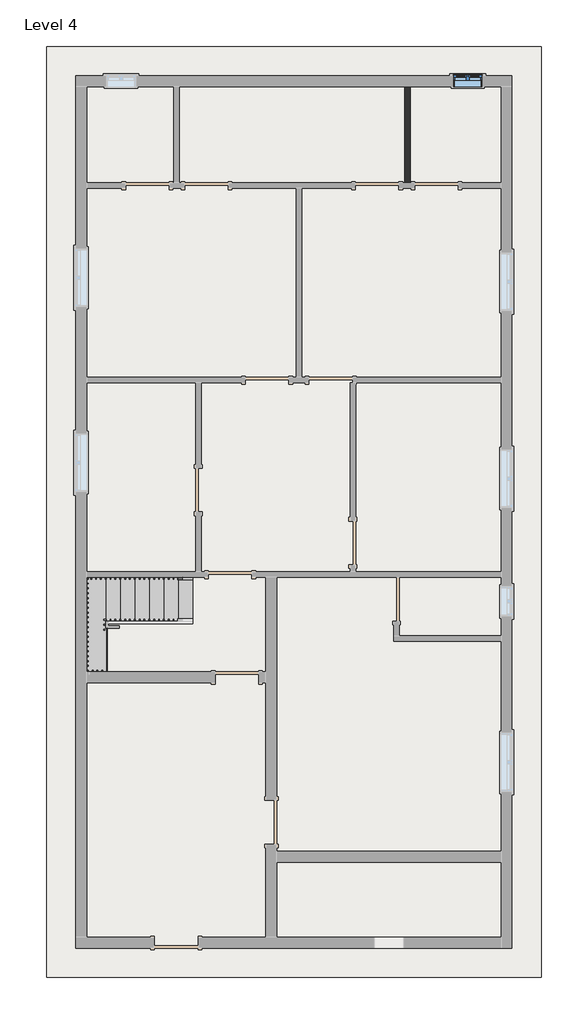
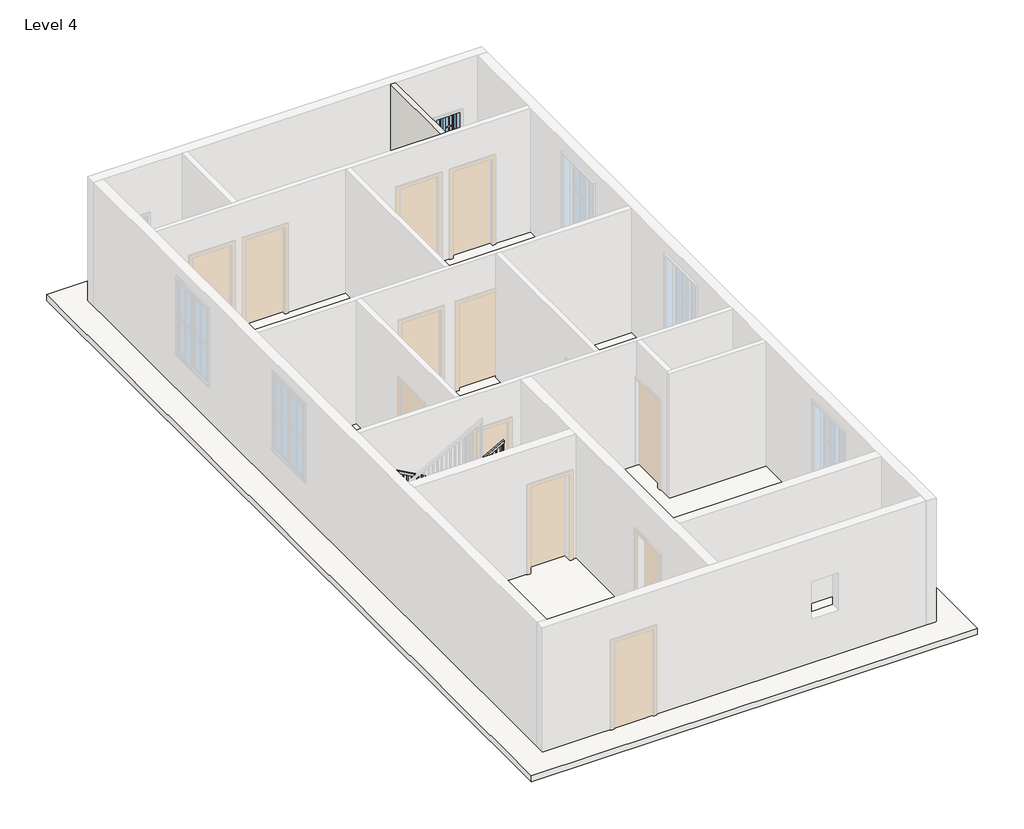
# One storey, part 2 of 3: 1 railing, 1 slab, 1 stair flight, 1 wall, 1 window.
"""IFC4 building model written with IfcOpenShell, lengths in millimetres."""

from ifc_helpers import new_model, si_unit, frame, origin, place, context, project, spatial, polyline, outline, extrude, faceted_brep, transform, mapped, element, save
from components import stair_flight_ac649a0f, window_c417fced

model = new_model("IFC4")

# Units and contexts
model_context = context("Model", 3, world=origin())
ifc_project = project(units=[si_unit("LENGTHUNIT", "METRE", prefix="MILLI")], contexts=[model_context])

# Site, building, storey
site = spatial("IfcSite", under=ifc_project)
building = spatial("IfcBuilding", under=site)
storey = spatial("IfcBuildingStorey", under=building, Name="Level 4", Elevation=9144.0)

# Railing
placement = place(None, origin())
element("IfcRailing", 1, ObjectType="Handrail - Rectangular", at=placement, inside=storey, context=model_context, shape_type="SolidModel", body=[
    faceted_brep([(3727.9146873, 3657.6, 10227.7333333), (3727.9146873, 3657.6, 10169.620221), (3727.9146873, 3708.4, 10169.620221), (3727.9146873, 3708.4, 10227.7333333), (1899.1146873, 3657.6, 11243.7333333), (1885.9510851, 3657.6, 11192.9333333), (1885.9510851, 3708.4, 11192.9333333), (1899.1146873, 3708.4, 11243.7333333), (1549.4, 3657.6, 11243.7333333), (1549.4, 3657.6, 11192.9333333), (1498.6, 3708.4, 11192.9333333), (1498.6, 3708.4, 11243.7333333), (1549.4, 1778.0, 11243.7333333), (1549.4, 1778.0, 11192.9333333), (1498.6, 1727.2, 11192.9333333), (1498.6, 1727.2, 11243.7333333), (1594.3146873, 1778.0, 11243.7333333), (1607.4782895, 1778.0, 11192.9333333), (1607.4782895, 1727.2, 11192.9333333), (1594.3146873, 1727.2, 11243.7333333), (3727.9146873, 1778.0, 12429.0666667), (3727.9146873, 1727.2, 12429.0666667), (3727.9146873, 1727.2, 12370.9535543), (3727.9146873, 1778.0, 12370.9535543)], [[[0, 1, 2, 3]], [[1, 0, 4, 5]], [[2, 1, 5, 6]], [[3, 2, 6, 7]], [[0, 3, 7, 4]], [[5, 4, 8, 9]], [[6, 5, 9, 10]], [[7, 6, 10, 11]], [[4, 7, 11, 8]], [[9, 8, 12, 13]], [[10, 9, 13, 14]], [[11, 10, 14, 15]], [[8, 11, 15, 12]], [[13, 12, 16, 17]], [[14, 13, 17, 18]], [[15, 14, 18, 19]], [[12, 15, 19, 16]], [[20, 21, 22, 23]], [[17, 16, 20, 23]], [[18, 17, 23, 22]], [[19, 18, 22, 21]], [[16, 19, 21, 20]]]),
    extrude(outline(polyline([(12337.1815058, 3667.125), (12326.5981725, 3648.075), (11345.3333333, 3648.075), (11345.3333333, 3667.125), (12337.1815058, 3667.125)])), frame((0.0, 1743.075, 0.0), z_axis=(0.0, 1.0, 0.0), x_axis=(0.0, 0.0, 1.0)), (0.0, 0.0, 1.0), 19.05),
    extrude(outline(polyline([(12280.7370614, 3565.525), (12270.153728, 3546.475), (11345.3333333, 3546.475), (11345.3333333, 3565.525), (12280.7370614, 3565.525)])), frame((0.0, 1743.075, 0.0), z_axis=(0.0, 1.0, 0.0), x_axis=(0.0, 0.0, 1.0)), (0.0, 0.0, 1.0), 19.05),
    extrude(outline(polyline([(12224.2926169, 3463.925), (12213.7092836, 3444.875), (11345.3333333, 3444.875), (11345.3333333, 3463.925), (12224.2926169, 3463.925)])), frame((0.0, 1743.075, 0.0), z_axis=(0.0, 1.0, 0.0), x_axis=(0.0, 0.0, 1.0)), (0.0, 0.0, 1.0), 19.05),
    extrude(outline(polyline([(12167.8481725, 3362.325), (12157.2648391, 3343.275), (11176.0, 3343.275), (11176.0, 3362.325), (12167.8481725, 3362.325)])), frame((0.0, 1743.075, 0.0), z_axis=(0.0, 1.0, 0.0), x_axis=(0.0, 0.0, 1.0)), (0.0, 0.0, 1.0), 19.05),
    extrude(outline(polyline([(12111.403728, 3260.725), (12100.8203947, 3241.675), (11176.0, 3241.675), (11176.0, 3260.725), (12111.403728, 3260.725)])), frame((0.0, 1743.075, 0.0), z_axis=(0.0, 1.0, 0.0), x_axis=(0.0, 0.0, 1.0)), (0.0, 0.0, 1.0), 19.05),
    extrude(outline(polyline([(12054.9592836, 3159.125), (12044.3759503, 3140.075), (11176.0, 3140.075), (11176.0, 3159.125), (12054.9592836, 3159.125)])), frame((0.0, 1743.075, 0.0), z_axis=(0.0, 1.0, 0.0), x_axis=(0.0, 0.0, 1.0)), (0.0, 0.0, 1.0), 19.05),
    extrude(outline(polyline([(11998.5148391, 3057.525), (11987.9315058, 3038.475), (11006.6666667, 3038.475), (11006.6666667, 3057.525), (11998.5148391, 3057.525)])), frame((0.0, 1743.075, 0.0), z_axis=(0.0, 1.0, 0.0), x_axis=(0.0, 0.0, 1.0)), (0.0, 0.0, 1.0), 19.05),
    extrude(outline(polyline([(11942.0703947, 2955.925), (11931.4870614, 2936.875), (11006.6666667, 2936.875), (11006.6666667, 2955.925), (11942.0703947, 2955.925)])), frame((0.0, 1743.075, 0.0), z_axis=(0.0, 1.0, 0.0), x_axis=(0.0, 0.0, 1.0)), (0.0, 0.0, 1.0), 19.05),
    extrude(outline(polyline([(11885.6259503, 2854.325), (11875.0426169, 2835.275), (11006.6666667, 2835.275), (11006.6666667, 2854.325), (11885.6259503, 2854.325)])), frame((0.0, 1743.075, 0.0), z_axis=(0.0, 1.0, 0.0), x_axis=(0.0, 0.0, 1.0)), (0.0, 0.0, 1.0), 19.05),
    extrude(outline(polyline([(11829.1815058, 2752.725), (11818.5981725, 2733.675), (10837.3333333, 2733.675), (10837.3333333, 2752.725), (11829.1815058, 2752.725)])), frame((0.0, 1743.075, 0.0), z_axis=(0.0, 1.0, 0.0), x_axis=(0.0, 0.0, 1.0)), (0.0, 0.0, 1.0), 19.05),
    extrude(outline(polyline([(11772.7370614, 2651.125), (11762.153728, 2632.075), (10837.3333333, 2632.075), (10837.3333333, 2651.125), (11772.7370614, 2651.125)])), frame((0.0, 1743.075, 0.0), z_axis=(0.0, 1.0, 0.0), x_axis=(0.0, 0.0, 1.0)), (0.0, 0.0, 1.0), 19.05),
    extrude(outline(polyline([(11716.2926169, 2549.525), (11705.7092836, 2530.475), (10837.3333333, 2530.475), (10837.3333333, 2549.525), (11716.2926169, 2549.525)])), frame((0.0, 1743.075, 0.0), z_axis=(0.0, 1.0, 0.0), x_axis=(0.0, 0.0, 1.0)), (0.0, 0.0, 1.0), 19.05),
    extrude(outline(polyline([(11659.8481725, 2447.925), (11649.2648391, 2428.875), (10668.0, 2428.875), (10668.0, 2447.925), (11659.8481725, 2447.925)])), frame((0.0, 1743.075, 0.0), z_axis=(0.0, 1.0, 0.0), x_axis=(0.0, 0.0, 1.0)), (0.0, 0.0, 1.0), 19.05),
    extrude(outline(polyline([(11603.403728, 2346.325), (11592.8203947, 2327.275), (10668.0, 2327.275), (10668.0, 2346.325), (11603.403728, 2346.325)])), frame((0.0, 1743.075, 0.0), z_axis=(0.0, 1.0, 0.0), x_axis=(0.0, 0.0, 1.0)), (0.0, 0.0, 1.0), 19.05),
    extrude(outline(polyline([(11546.9592836, 2244.725), (11536.3759503, 2225.675), (10668.0, 2225.675), (10668.0, 2244.725), (11546.9592836, 2244.725)])), frame((0.0, 1743.075, 0.0), z_axis=(0.0, 1.0, 0.0), x_axis=(0.0, 0.0, 1.0)), (0.0, 0.0, 1.0), 19.05),
    extrude(outline(polyline([(11490.5148391, 2143.125), (11479.9315058, 2124.075), (10498.6666667, 2124.075), (10498.6666667, 2143.125), (11490.5148391, 2143.125)])), frame((0.0, 1743.075, 0.0), z_axis=(0.0, 1.0, 0.0), x_axis=(0.0, 0.0, 1.0)), (0.0, 0.0, 1.0), 19.05),
    extrude(outline(polyline([(11434.0703947, 2041.525), (11423.4870614, 2022.475), (10498.6666667, 2022.475), (10498.6666667, 2041.525), (11434.0703947, 2041.525)])), frame((0.0, 1743.075, 0.0), z_axis=(0.0, 1.0, 0.0), x_axis=(0.0, 0.0, 1.0)), (0.0, 0.0, 1.0), 19.05),
    extrude(outline(polyline([(11377.6259503, 1939.925), (11367.0426169, 1920.875), (10498.6666667, 1920.875), (10498.6666667, 1939.925), (11377.6259503, 1939.925)])), frame((0.0, 1743.075, 0.0), z_axis=(0.0, 1.0, 0.0), x_axis=(0.0, 0.0, 1.0)), (0.0, 0.0, 1.0), 19.05),
    extrude(outline(polyline([(11321.1815058, 1838.325), (11310.5981725, 1819.275), (10329.3333333, 1819.275), (10329.3333333, 1838.325), (11321.1815058, 1838.325)])), frame((0.0, 1743.075, 0.0), z_axis=(0.0, 1.0, 0.0), x_axis=(0.0, 0.0, 1.0)), (0.0, 0.0, 1.0), 19.05),
    extrude(outline(polyline([(11264.7370614, 1736.725), (11254.153728, 1717.675), (10329.3333333, 1717.675), (10329.3333333, 1736.725), (11264.7370614, 1736.725)])), frame((0.0, 1743.075, 0.0), z_axis=(0.0, 1.0, 0.0), x_axis=(0.0, 0.0, 1.0)), (0.0, 0.0, 1.0), 19.05),
    extrude(outline(polyline([(11208.2926169, 1635.125), (11197.7092836, 1616.075), (10329.3333333, 1616.075), (10329.3333333, 1635.125), (11208.2926169, 1635.125)])), frame((0.0, 1743.075, 0.0), z_axis=(0.0, 1.0, 0.0), x_axis=(0.0, 0.0, 1.0)), (0.0, 0.0, 1.0), 19.05),
    extrude(outline(polyline([(1514.475, 1863.725), (1533.525, 1863.725), (1533.525, 1844.675), (1514.475, 1844.675), (1514.475, 1863.725)])), frame((0.0, 0.0, 10329.3333333), z_axis=(0.0, 0.0, 1.0), x_axis=(1.0, 0.0, 0.0)), (0.0, 0.0, 1.0), 863.6),
    extrude(outline(polyline([(1514.475, 1965.325), (1533.525, 1965.325), (1533.525, 1946.275), (1514.475, 1946.275), (1514.475, 1965.325)])), frame((0.0, 0.0, 10329.3333333), z_axis=(0.0, 0.0, 1.0), x_axis=(1.0, 0.0, 0.0)), (0.0, 0.0, 1.0), 863.6),
    extrude(outline(polyline([(1514.475, 2066.925), (1533.525, 2066.925), (1533.525, 2047.875), (1514.475, 2047.875), (1514.475, 2066.925)])), frame((0.0, 0.0, 10329.3333333), z_axis=(0.0, 0.0, 1.0), x_axis=(1.0, 0.0, 0.0)), (0.0, 0.0, 1.0), 863.6),
    extrude(outline(polyline([(1514.475, 2168.525), (1533.525, 2168.525), (1533.525, 2149.475), (1514.475, 2149.475), (1514.475, 2168.525)])), frame((0.0, 0.0, 10329.3333333), z_axis=(0.0, 0.0, 1.0), x_axis=(1.0, 0.0, 0.0)), (0.0, 0.0, 1.0), 863.6),
    extrude(outline(polyline([(1514.475, 2270.125), (1533.525, 2270.125), (1533.525, 2251.075), (1514.475, 2251.075), (1514.475, 2270.125)])), frame((0.0, 0.0, 10329.3333333), z_axis=(0.0, 0.0, 1.0), x_axis=(1.0, 0.0, 0.0)), (0.0, 0.0, 1.0), 863.6),
    extrude(outline(polyline([(1514.475, 2371.725), (1533.525, 2371.725), (1533.525, 2352.675), (1514.475, 2352.675), (1514.475, 2371.725)])), frame((0.0, 0.0, 10329.3333333), z_axis=(0.0, 0.0, 1.0), x_axis=(1.0, 0.0, 0.0)), (0.0, 0.0, 1.0), 863.6),
    extrude(outline(polyline([(1514.475, 2473.325), (1533.525, 2473.325), (1533.525, 2454.275), (1514.475, 2454.275), (1514.475, 2473.325)])), frame((0.0, 0.0, 10329.3333333), z_axis=(0.0, 0.0, 1.0), x_axis=(1.0, 0.0, 0.0)), (0.0, 0.0, 1.0), 863.6),
    extrude(outline(polyline([(1514.475, 2574.925), (1533.525, 2574.925), (1533.525, 2555.875), (1514.475, 2555.875), (1514.475, 2574.925)])), frame((0.0, 0.0, 10329.3333333), z_axis=(0.0, 0.0, 1.0), x_axis=(1.0, 0.0, 0.0)), (0.0, 0.0, 1.0), 863.6),
    extrude(outline(polyline([(1514.475, 2676.525), (1533.525, 2676.525), (1533.525, 2657.475), (1514.475, 2657.475), (1514.475, 2676.525)])), frame((0.0, 0.0, 10329.3333333), z_axis=(0.0, 0.0, 1.0), x_axis=(1.0, 0.0, 0.0)), (0.0, 0.0, 1.0), 863.6),
    extrude(outline(polyline([(1514.475, 2778.125), (1533.525, 2778.125), (1533.525, 2759.075), (1514.475, 2759.075), (1514.475, 2778.125)])), frame((0.0, 0.0, 10329.3333333), z_axis=(0.0, 0.0, 1.0), x_axis=(1.0, 0.0, 0.0)), (0.0, 0.0, 1.0), 863.6),
    extrude(outline(polyline([(1514.475, 2879.725), (1533.525, 2879.725), (1533.525, 2860.675), (1514.475, 2860.675), (1514.475, 2879.725)])), frame((0.0, 0.0, 10329.3333333), z_axis=(0.0, 0.0, 1.0), x_axis=(1.0, 0.0, 0.0)), (0.0, 0.0, 1.0), 863.6),
    extrude(outline(polyline([(1514.475, 2981.325), (1533.525, 2981.325), (1533.525, 2962.275), (1514.475, 2962.275), (1514.475, 2981.325)])), frame((0.0, 0.0, 10329.3333333), z_axis=(0.0, 0.0, 1.0), x_axis=(1.0, 0.0, 0.0)), (0.0, 0.0, 1.0), 863.6),
    extrude(outline(polyline([(1514.475, 3082.925), (1533.525, 3082.925), (1533.525, 3063.875), (1514.475, 3063.875), (1514.475, 3082.925)])), frame((0.0, 0.0, 10329.3333333), z_axis=(0.0, 0.0, 1.0), x_axis=(1.0, 0.0, 0.0)), (0.0, 0.0, 1.0), 863.6),
    extrude(outline(polyline([(1514.475, 3184.525), (1533.525, 3184.525), (1533.525, 3165.475), (1514.475, 3165.475), (1514.475, 3184.525)])), frame((0.0, 0.0, 10329.3333333), z_axis=(0.0, 0.0, 1.0), x_axis=(1.0, 0.0, 0.0)), (0.0, 0.0, 1.0), 863.6),
    extrude(outline(polyline([(1514.475, 3286.125), (1533.525, 3286.125), (1533.525, 3267.075), (1514.475, 3267.075), (1514.475, 3286.125)])), frame((0.0, 0.0, 10329.3333333), z_axis=(0.0, 0.0, 1.0), x_axis=(1.0, 0.0, 0.0)), (0.0, 0.0, 1.0), 863.6),
    extrude(outline(polyline([(1514.475, 3387.725), (1533.525, 3387.725), (1533.525, 3368.675), (1514.475, 3368.675), (1514.475, 3387.725)])), frame((0.0, 0.0, 10329.3333333), z_axis=(0.0, 0.0, 1.0), x_axis=(1.0, 0.0, 0.0)), (0.0, 0.0, 1.0), 863.6),
    extrude(outline(polyline([(1514.475, 3489.325), (1533.525, 3489.325), (1533.525, 3470.275), (1514.475, 3470.275), (1514.475, 3489.325)])), frame((0.0, 0.0, 10329.3333333), z_axis=(0.0, 0.0, 1.0), x_axis=(1.0, 0.0, 0.0)), (0.0, 0.0, 1.0), 863.6),
    extrude(outline(polyline([(1514.475, 3590.925), (1533.525, 3590.925), (1533.525, 3571.875), (1514.475, 3571.875), (1514.475, 3590.925)])), frame((0.0, 0.0, 10329.3333333), z_axis=(0.0, 0.0, 1.0), x_axis=(1.0, 0.0, 0.0)), (0.0, 0.0, 1.0), 863.6),
    extrude(outline(polyline([(1603.8396873, 3692.525), (1603.8396873, 3673.475), (1584.7896873, 3673.475), (1584.7896873, 3692.525), (1603.8396873, 3692.525)])), frame((0.0, 0.0, 10329.3333333), z_axis=(0.0, 0.0, 1.0), x_axis=(1.0, 0.0, 0.0)), (0.0, 0.0, 1.0), 863.6),
    extrude(outline(polyline([(1705.4396873, 3692.525), (1705.4396873, 3673.475), (1686.3896873, 3673.475), (1686.3896873, 3692.525), (1705.4396873, 3692.525)])), frame((0.0, 0.0, 10329.3333333), z_axis=(0.0, 0.0, 1.0), x_axis=(1.0, 0.0, 0.0)), (0.0, 0.0, 1.0), 863.6),
    extrude(outline(polyline([(1807.0396873, 3692.525), (1807.0396873, 3673.475), (1787.9896873, 3673.475), (1787.9896873, 3692.525), (1807.0396873, 3692.525)])), frame((0.0, 0.0, 10329.3333333), z_axis=(0.0, 0.0, 1.0), x_axis=(1.0, 0.0, 0.0)), (0.0, 0.0, 1.0), 863.6),
    extrude(outline(polyline([(11180.3285543, 1908.6396873), (11190.9118876, 1889.5896873), (10329.3333333, 1889.5896873), (10329.3333333, 1908.6396873), (11180.3285543, 1908.6396873)])), frame((0.0, 3673.475, 0.0), z_axis=(0.0, 1.0, 0.0), x_axis=(0.0, 0.0, 1.0)), (0.0, 0.0, 1.0), 19.05),
    extrude(outline(polyline([(11123.8841099, 2010.2396873), (11134.4674432, 1991.1896873), (10160.0, 1991.1896873), (10160.0, 2010.2396873), (11123.8841099, 2010.2396873)])), frame((0.0, 3673.475, 0.0), z_axis=(0.0, 1.0, 0.0), x_axis=(0.0, 0.0, 1.0)), (0.0, 0.0, 1.0), 19.05),
    extrude(outline(polyline([(11067.4396654, 2111.8396873), (11078.0229988, 2092.7896873), (10160.0, 2092.7896873), (10160.0, 2111.8396873), (11067.4396654, 2111.8396873)])), frame((0.0, 3673.475, 0.0), z_axis=(0.0, 1.0, 0.0), x_axis=(0.0, 0.0, 1.0)), (0.0, 0.0, 1.0), 19.05),
    extrude(outline(polyline([(11010.995221, 2213.4396873), (11021.5785543, 2194.3896873), (10160.0, 2194.3896873), (10160.0, 2213.4396873), (11010.995221, 2213.4396873)])), frame((0.0, 3673.475, 0.0), z_axis=(0.0, 1.0, 0.0), x_axis=(0.0, 0.0, 1.0)), (0.0, 0.0, 1.0), 19.05),
    extrude(outline(polyline([(10954.5507765, 2315.0396873), (10965.1341099, 2295.9896873), (9990.6666667, 2295.9896873), (9990.6666667, 2315.0396873), (10954.5507765, 2315.0396873)])), frame((0.0, 3673.475, 0.0), z_axis=(0.0, 1.0, 0.0), x_axis=(0.0, 0.0, 1.0)), (0.0, 0.0, 1.0), 19.05),
    extrude(outline(polyline([(10898.1063321, 2416.6396873), (10908.6896654, 2397.5896873), (9990.6666667, 2397.5896873), (9990.6666667, 2416.6396873), (10898.1063321, 2416.6396873)])), frame((0.0, 3673.475, 0.0), z_axis=(0.0, 1.0, 0.0), x_axis=(0.0, 0.0, 1.0)), (0.0, 0.0, 1.0), 19.05),
    extrude(outline(polyline([(10841.6618876, 2518.2396873), (10852.245221, 2499.1896873), (9990.6666667, 2499.1896873), (9990.6666667, 2518.2396873), (10841.6618876, 2518.2396873)])), frame((0.0, 3673.475, 0.0), z_axis=(0.0, 1.0, 0.0), x_axis=(0.0, 0.0, 1.0)), (0.0, 0.0, 1.0), 19.05),
    extrude(outline(polyline([(10785.2174432, 2619.8396873), (10795.8007765, 2600.7896873), (9821.3333333, 2600.7896873), (9821.3333333, 2619.8396873), (10785.2174432, 2619.8396873)])), frame((0.0, 3673.475, 0.0), z_axis=(0.0, 1.0, 0.0), x_axis=(0.0, 0.0, 1.0)), (0.0, 0.0, 1.0), 19.05),
    extrude(outline(polyline([(10728.7729988, 2721.4396873), (10739.3563321, 2702.3896873), (9821.3333333, 2702.3896873), (9821.3333333, 2721.4396873), (10728.7729988, 2721.4396873)])), frame((0.0, 3673.475, 0.0), z_axis=(0.0, 1.0, 0.0), x_axis=(0.0, 0.0, 1.0)), (0.0, 0.0, 1.0), 19.05),
    extrude(outline(polyline([(10672.3285543, 2823.0396873), (10682.9118876, 2803.9896873), (9821.3333333, 2803.9896873), (9821.3333333, 2823.0396873), (10672.3285543, 2823.0396873)])), frame((0.0, 3673.475, 0.0), z_axis=(0.0, 1.0, 0.0), x_axis=(0.0, 0.0, 1.0)), (0.0, 0.0, 1.0), 19.05),
    extrude(outline(polyline([(10615.8841099, 2924.6396873), (10626.4674432, 2905.5896873), (9652.0, 2905.5896873), (9652.0, 2924.6396873), (10615.8841099, 2924.6396873)])), frame((0.0, 3673.475, 0.0), z_axis=(0.0, 1.0, 0.0), x_axis=(0.0, 0.0, 1.0)), (0.0, 0.0, 1.0), 19.05),
    extrude(outline(polyline([(10559.4396654, 3026.2396873), (10570.0229988, 3007.1896873), (9652.0, 3007.1896873), (9652.0, 3026.2396873), (10559.4396654, 3026.2396873)])), frame((0.0, 3673.475, 0.0), z_axis=(0.0, 1.0, 0.0), x_axis=(0.0, 0.0, 1.0)), (0.0, 0.0, 1.0), 19.05),
    extrude(outline(polyline([(10502.995221, 3127.8396873), (10513.5785543, 3108.7896873), (9652.0, 3108.7896873), (9652.0, 3127.8396873), (10502.995221, 3127.8396873)])), frame((0.0, 3673.475, 0.0), z_axis=(0.0, 1.0, 0.0), x_axis=(0.0, 0.0, 1.0)), (0.0, 0.0, 1.0), 19.05),
    extrude(outline(polyline([(10446.5507765, 3229.4396873), (10457.1341099, 3210.3896873), (9482.6666667, 3210.3896873), (9482.6666667, 3229.4396873), (10446.5507765, 3229.4396873)])), frame((0.0, 3673.475, 0.0), z_axis=(0.0, 1.0, 0.0), x_axis=(0.0, 0.0, 1.0)), (0.0, 0.0, 1.0), 19.05),
    extrude(outline(polyline([(10390.1063321, 3331.0396873), (10400.6896654, 3311.9896873), (9482.6666667, 3311.9896873), (9482.6666667, 3331.0396873), (10390.1063321, 3331.0396873)])), frame((0.0, 3673.475, 0.0), z_axis=(0.0, 1.0, 0.0), x_axis=(0.0, 0.0, 1.0)), (0.0, 0.0, 1.0), 19.05),
    extrude(outline(polyline([(10333.6618876, 3432.6396873), (10344.245221, 3413.5896873), (9482.6666667, 3413.5896873), (9482.6666667, 3432.6396873), (10333.6618876, 3432.6396873)])), frame((0.0, 3673.475, 0.0), z_axis=(0.0, 1.0, 0.0), x_axis=(0.0, 0.0, 1.0)), (0.0, 0.0, 1.0), 19.05),
    extrude(outline(polyline([(10277.2174432, 3534.2396873), (10287.8007765, 3515.1896873), (9313.3333333, 3515.1896873), (9313.3333333, 3534.2396873), (10277.2174432, 3534.2396873)])), frame((0.0, 3673.475, 0.0), z_axis=(0.0, 1.0, 0.0), x_axis=(0.0, 0.0, 1.0)), (0.0, 0.0, 1.0), 19.05),
    extrude(outline(polyline([(10220.7729988, 3635.8396873), (10231.3563321, 3616.7896873), (9313.3333333, 3616.7896873), (9313.3333333, 3635.8396873), (10220.7729988, 3635.8396873)])), frame((0.0, 3673.475, 0.0), z_axis=(0.0, 1.0, 0.0), x_axis=(0.0, 0.0, 1.0)), (0.0, 0.0, 1.0), 19.05),
    extrude(outline(polyline([(1514.475, 1762.125), (1533.525, 1762.125), (1533.525, 1743.075), (1514.475, 1743.075), (1514.475, 1762.125)])), frame((0.0, 0.0, 10329.3333333), z_axis=(0.0, 0.0, 1.0), x_axis=(1.0, 0.0, 0.0)), (0.0, 0.0, 1.0), 863.6),
    extrude(outline(polyline([(1533.525, 3692.525), (1533.525, 3673.475), (1514.475, 3673.475), (1514.475, 3692.525), (1533.525, 3692.525)])), frame((0.0, 0.0, 10329.3333333), z_axis=(0.0, 0.0, 1.0), x_axis=(1.0, 0.0, 0.0)), (0.0, 0.0, 1.0), 863.6),
    extrude(outline(polyline([(12370.9535543, 3727.9146873), (12360.370221, 3708.8646873), (11345.3333333, 3708.8646873), (11345.3333333, 3727.9146873), (12370.9535543, 3727.9146873)])), frame((0.0, 1743.075, 0.0), z_axis=(0.0, 1.0, 0.0), x_axis=(0.0, 0.0, 1.0)), (0.0, 0.0, 1.0), 19.05),
    extrude(outline(polyline([(10169.620221, 3727.9146873), (10180.2035543, 3708.8646873), (9313.3333333, 3708.8646873), (9313.3333333, 3727.9146873), (10169.620221, 3727.9146873)])), frame((0.0, 3673.475, 0.0), z_axis=(0.0, 1.0, 0.0), x_axis=(0.0, 0.0, 1.0)), (0.0, 0.0, 1.0), 19.05),
])

# Slab
element("IfcSlab", 2, ObjectType="Generic - 12\"", at=placement, inside=storey, context=model_context, shape_type="SweptSolid", body=[
    extrude(outline(polyline([(11023.6, 14833.6), (11023.6, -4673.6), (660.4, -4673.6), (660.4, 14833.6), (11023.6, 14833.6)])), frame((0.0, 0.0, 8991.6), z_axis=(0.0, 0.0, 1.0), x_axis=(1.0, 0.0, 0.0)), (0.0, 0.0, 1.0), 152.4),
])

# Stair flight
stair_flight_shape = stair_flight_ac649a0f(model_context)
element("IfcStairFlight", 3, ObjectType="2\" Tread 1\" Nosing 1/4\" Riser", at=placement, inside=storey, context=model_context, shape_type="MappedRepresentation", body=[
    mapped(stair_flight_shape, transform((0.0, 0.0, 0.0), x_axis=(1.0, 0.0, 0.0), y_axis=(0.0, 1.0, 0.0), z_axis=(0.0, 0.0, 1.0))),
])

# Wall
element("IfcWall", 4, ObjectType="Generic - 5\"", at=placement, inside=storey, context=model_context, shape_type="SweptSolid", body=[
    extrude(outline(polyline([(8166.1, 11976.1), (8166.1, 13995.4), (8280.4, 13995.4), (8280.4, 11976.1), (8166.1, 11976.1)])), frame((0.0, 0.0, 9144.0), z_axis=(0.0, 0.0, 1.0), x_axis=(1.0, 0.0, 0.0)), (0.0, 0.0, 1.0), 3048.0),
])

# Window
window_shape = window_c417fced(model_context)
element("IfcWindow", 5, ObjectType="Window-Casement-Double : 24\" x 36\"", at=placement, inside=storey, context=model_context, shape_type="MappedRepresentation", body=[
    mapped(window_shape, transform((9486.9, 14109.7, 9144.0), x_axis=(1.0, 0.0, 0.0), y_axis=(0.0, 1.0, 0.0), z_axis=(0.0, 0.0, 1.0))),
])

save(model, "model.ifc")

# Revit data of these elements
# Type "Handrail - Rectangular"
#   Assembly Code = "C2010400"
#   built-in parameter 1008612 = 0.0416667 (stored number, unit not read)
#   built-in parameter 1008611 = 0.0416667 (stored number, unit not read)
#   built-in parameter 1008609 = 0.333333 (stored number, unit not read)
#   built-in parameter 1008604 = 0.166667 (stored number, unit not read)
#   built-in parameter 1008603 = 0.166667 (stored number, unit not read)
#   Railing Height = 3' - 0"
#   built-in parameter 1008630 = 2
#   built-in parameter 1008610 = 2
#   built-in parameter 1008618 = Baluster - Square : 3/4"
# Type "Generic - 12\""
#   Assembly Code = "B1010"
#   Function = 0
#   Layers, outside or top first: 0' - 6" "Door - Panel" (function 1)
# Type "Generic - 5\""
#   Assembly Code = "B2010"
#   Layers, outside or top first: 0' - 4 1/2" no material (function 1)
# Type "Window-Casement-Double : 24\" x 36\""
#   Type Mark = "14"
#   Fire Rating = "0.5h"
#   Assembly Code = "B2020100"
#   Analytic Construction = "Double glazing - domestic"
#   Frame Extension [instance default] = 0' - 0 1/4"
#   Window Inset [instance default] = 0' - 0"
#   Wall Thickness [instance default] = 0' - 6"
#   Interior Wall Closure [instance default] = 0' - 2 1/4"
#   Half Width = 1' - 0"
#   Visual Light Transmittance = 0.81
#   Thermal Resistance (R) = 1.8146 (h·ft²·°F)/BTU
#   Solar Heat Gain Coefficient = 0.76
#   Rough Width = 2' - 0 1/2"
#   Rough Height = 3' - 0 1/2"
#   Height = 3' - 0"
#   Heat Transfer Coefficient (U) = 0.5511 BTU/(h·ft²·°F)
#   Exterior Wall Closure [instance default] = 0' - 1 1/4"
#   Extension Jamb [instance default] = 0' - 2 1/4"
#   Default Sill Height = 3' - 0"
#   Width = 2' - 0"
#   Define Thermal Properties by = 0
#   Muntin Visibility = yes
#   Interior Trim Visibility [instance default] = yes
#   Exterior Trim Visibility [instance default] = yes
#   Extension Jamb Visibility [instance default] = yes
#   Interior Trim Material = Wood - Stained
#   Muntin Pattern = Muntin Pattern_2x2 : Muntin Pattern_2x2
#   Interior Trim = Trim-Window-Interior-Flat : Picture Frame
#   Interior Frame Material = Wood - Stained
#   Glass Panel Material = Glass
#   Exterior Trim Material = Clad - White
#   Exterior Trim = Trim-Window-Exterior-Flat : with Sill
#   Exterior Frame Material = Clad - White
#   Wall Closure = (empty or 0)
# Element 1 (IfcRailing, "Handrail - Rectangular")
#   Phase Created = New Construction
# Element 2 (IfcSlab, "Generic - 12\"")
#   Height Offset From Level = 0' - 0"
#   Phase Created = New Construction
#   Materials on its faces: "Door - Panel"
# Element 3 (IfcStairFlight, "2\" Tread 1\" Nosing 1/4\" Riser")
#   Phase Created = New Construction
# Element 4 (IfcWall, "Generic - 5\"")
#   Top Offset = 0' - 0"
#   Base Offset = 0' - 0"
#   wall height = 10' - 0"
#   Phase Created = New Construction
#   Base Constraint = Level 4
#   Top Constraint = Level 5
#   Materials on its faces: "Default Wall"
# Element 5 (IfcWindow, "Window-Casement-Double : 24\" x 36\"")
#   Mark = "31"
#   Window Inset = 0' - 0"
#   Interior Wall Closure = 0' - 2 1/4"
#   Frame Extension = 0' - 0 1/4"
#   Exterior Wall Closure = 0' - 1 1/4"
#   Interior Trim Visibility = yes
#   Exterior Trim Visibility = yes
#   Phase Created = New Construction
#   Materials on its faces: "Wood - Stained", "Glass", "Clad - White"
# Materials
#   "Door - Panel": class "Wood", colour RGB 210 159 95, transparency 0, Cost = 0
#   "Wood - Stained": class "Wood", colour RGB 224 178 126, transparency 0, Cost = 0
#   "Glass": class "Glass", colour RGB 0 128 192, transparency 0.75, Description = "Soda Lime Glass", Cost = 0
#   "Clad - White": class "Wood", colour RGB 242 242 238, transparency 0, Cost = 0
#   "Default Wall": colour RGB 128 128 128, transparency 0, Cost = 0
